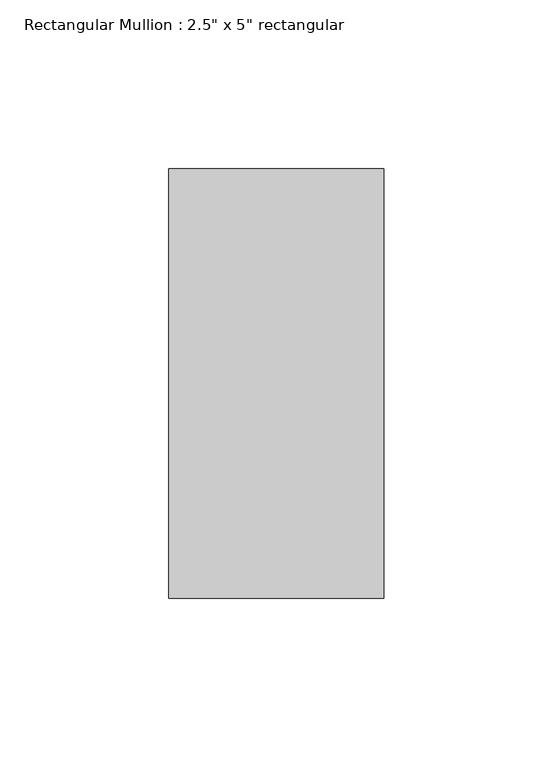
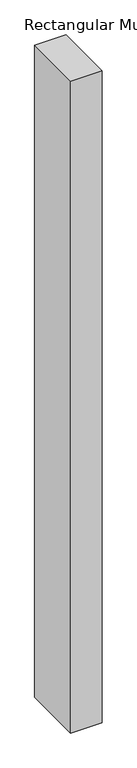
"""IFC4 building model written with IfcOpenShell, lengths in millimetres: member geometry."""

from ifc_helpers import new_model, si_unit, frame, origin, place, context, project, spatial, polyline, outline, extrude, source, transform, mapped, element, save


def member_1bb00157(model_context):
    return source(origin(), model_context, "Body", "SweptSolid", [
        extrude(outline(polyline([(31.75, 63.5), (31.75, -63.5), (-31.75, -63.5), (-31.75, 63.5), (31.75, 63.5)])), frame((0.0, 0.0, -1401.8499484), z_axis=(0.0, 0.0, 1.0), x_axis=(1.0, 0.0, 0.0)), (0.0, 0.0, 1.0), 1401.8499484),
    ])


if __name__ == "__main__":
    model = new_model("IFC4")
    model_context = context("Model", 3, world=origin())
    ifc_project = project(units=[si_unit("LENGTHUNIT", "METRE", prefix="MILLI")], contexts=[model_context])
    site = spatial("IfcSite", under=ifc_project)
    building = spatial("IfcBuilding", under=site)
    placement = place(None, origin())
    member_shape = member_1bb00157(model_context)
    element("IfcMember", 1, ObjectType="Rectangular Mullion : 2.5\" x 5\" rectangular", at=placement, inside=building, context=model_context, shape_type="MappedRepresentation", body=[
        mapped(member_shape, transform((0.0, 0.0, 0.0), x_axis=(1.0, 0.0, 0.0), y_axis=(0.0, 1.0, 0.0), z_axis=(0.0, 0.0, 1.0))),
    ])
    save(model, "model.ifc")

# Revit data of these elements
# Type "Rectangular Mullion : 2.5\" x 5\" rectangular"
#   built-in parameter 1007304 = 0.416667 (stored number, unit not read)
#   built-in parameter 1007301 = 0.104167 (stored number, unit not read)
#   built-in parameter 1007300 = 0.104167 (stored number, unit not read)
# Element 1 (IfcMember, "Rectangular Mullion : 2.5\" x 5\" rectangular")
#   Materials on its faces: "Aluminum"
# Materials
#   "Aluminum": class "Metal", colour RGB 247 247 247, transparency 0, Description = "Aluminum 6061", Cost = 0
